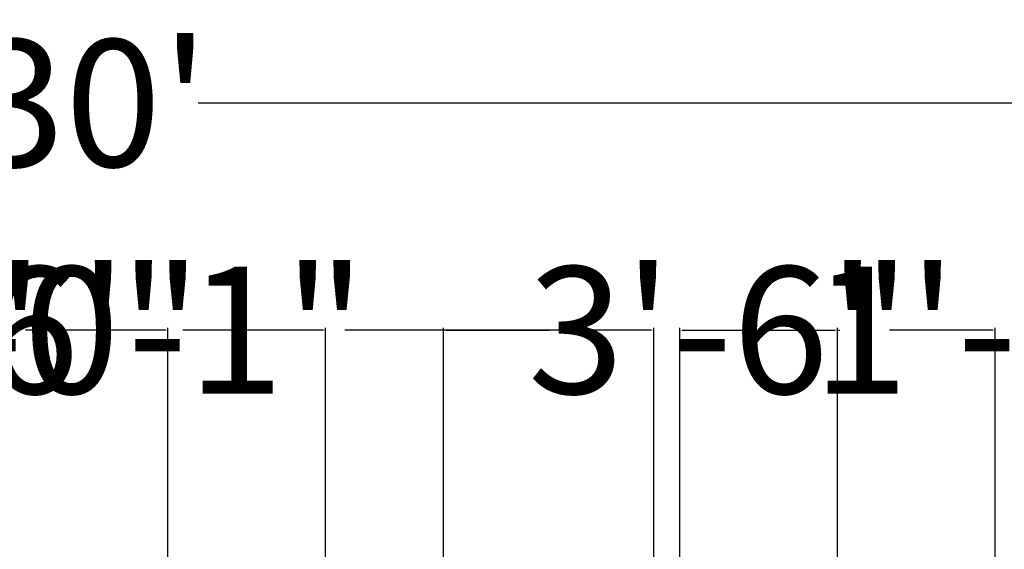
# Model space of a CAD drawing. Units: inches. Extents: x 2103 to 2702, y 2405 to 3142.
# Tile 5 of 7: x 2421 to 2496, y 3102 to 3142. Entities that reach past the tile are written whole.
import ezdxf

# ---------------------------------------------------------------- set-up
doc = ezdxf.new("R2010")
doc.units = ezdxf.units.IN
doc.layers.add('A-ANNO-DIMS', color=2, linetype='Continuous', lineweight=18)
doc.styles.get("Standard").update_dxf_attribs({"font": 'arial.ttf'})
doc.dimstyles.get("Standard").update_dxf_attribs({"dimtxt": 9.68, "dimasz": 0.18, "dimexe": 0.18, "dimexo": 0.0625, "dimgap": 0.09, "dimtad": 0, "dimtih": 1, "dimtoh": 1, "dimdec": 1, "dimzin": 0, "dimdsep": 46, "dimlunit": 3, "dimtxsty": 'Standard', "dimcen": 0.09, "dimadec": 0, "dimazin": 0, "dimtfac": 1, "dimtdec": 1, "dimtofl": 0, "dimtmove": 0, "dimatfit": 3, "dimfxl": 1, "dimtolj": 1, "dimtzin": 0, "dimarcsym": 0})

# ---------------------------------------------------------------- blocks, each defined once
blk = doc.blocks.new('*D15')
at = {"layer": 'A-ANNO-DIMS', "color": 0, "lineweight": -2, "transparency": 16777216}
for p, q in [((2246.430135310188, 3068.908174366427), (2246.430135310188, 3136.18297836625)), ((2606.430135310187, 3068.908174366427), (2606.430135310187, 3136.18297836625)), ((2246.610135310187, 3136.002978366251), (2418.129303113734, 3136.002978366251)), ((2606.250135310188, 3136.002978366251), (2434.730967506641, 3136.002978366251))]:
    blk.add_line(p, q, dxfattribs=at)
at = {"layer": 'A-ANNO-DIMS', "color": 0, "transparency": 16777216}
for points in [[(2246.610135310187, 3136.032978366251), (2246.610135310187, 3135.97297836625), (2246.430135310188, 3136.002978366251)], [(2606.250135310188, 3136.032978366251), (2606.250135310188, 3135.97297836625), (2606.430135310187, 3136.002978366251)]]:
    blk.add_solid(points, dxfattribs=at)
at = {"layer": 'Defpoints', "color": 0, "transparency": 16777216}
for p in [(2606.430135310187, 3136.002978366251), (2246.430135310188, 3068.845674366427), (2606.430135310187, 3068.845674366427)]:
    blk.add_point(p, dxfattribs=at)
at = {"layer": 'A-ANNO-DIMS', "color": 0, "transparency": 16777216, "insert": (2426.430135310188, 3136.002978366251), "char_height": 9.68, "attachment_point": 5}
blk.add_mtext("\\A1;30'", dxfattribs=at)
blk = doc.blocks.new('*D32')
at = {"layer": 'A-ANNO-DIMS', "color": 0, "lineweight": -2, "transparency": 16777216}
for p, q in [((2523.701954441973, 3069.816092044852), (2527.298623542507, 3072.777740503555)), ((2527.0452500719, 3072.802273835842), (2526.8652500719, 3072.802273835842)), ((2527.15967014106, 3072.663320434396), (2527.0452500719, 3072.802273835842)), ((2546.291633940058, 3049.429184449692), (2527.274090210219, 3072.524367032949)), ((2542.948338310131, 3046.443002658702), (2546.545007410664, 3049.404651117404))]:
    blk.add_line(p, q, dxfattribs=at)
at = {"layer": 'A-ANNO-DIMS', "color": 0, "transparency": 16777216}
for points in [[(2527.297249110461, 3072.543437044476), (2527.250931309978, 3072.505297021422), (2527.15967014106, 3072.663320434396)], [(2546.3147928403, 3049.448254461218), (2546.268475039817, 3049.410114438165), (2546.406054009218, 3049.290231048245)]]:
    blk.add_solid(points, dxfattribs=at)
at = {"layer": 'Defpoints', "color": 0, "transparency": 16777216}
for p in [(2527.15967014106, 3072.663320434396), (2523.653706733137, 3069.776362854172), (2542.900090601295, 3046.403273468022)]:
    blk.add_point(p, dxfattribs=at)
at = {"layer": 'A-ANNO-DIMS', "color": 0, "transparency": 16777216, "insert": (2430.028074082815, 3072.802273835842), "char_height": 9.68, "attachment_point": 5}
blk.add_mtext('\\A1;SINK ENVELOPE 2\'-6 1/2" TYP.', dxfattribs=at)
blk = doc.blocks.new('*D40')
at = {"layer": 'A-ANNO-DIMS', "color": 0, "lineweight": -2, "transparency": 16777216}
for p, q in [((2396.430135, 2906.908174), (2396.430135, 3118.895223)), ((2396.610135, 3118.715223000001), (2407.279400801501, 3118.715223000001)), ((2444.25014, 3118.715223000001), (2433.580874198499, 3118.715223000001)), ((2444.43014, 2842.908175), (2444.43014, 3118.895223))]:
    blk.add_line(p, q, dxfattribs=at)
at = {"layer": 'A-ANNO-DIMS', "color": 0, "transparency": 16777216}
for points in [[(2396.610135, 3118.745223000001), (2396.610135, 3118.685223), (2396.430135, 3118.715223000001)], [(2444.25014, 3118.745223000001), (2444.25014, 3118.685223), (2444.43014, 3118.715223000001)]]:
    blk.add_solid(points, dxfattribs=at)
at = {"layer": 'Defpoints', "color": 0, "transparency": 16777216}
for p in [(2444.43014, 3118.715223000001), (2396.430135, 2906.845674), (2444.43014, 2842.845675)]:
    blk.add_point(p, dxfattribs=at)
at = {"layer": 'A-ANNO-DIMS', "color": 0, "transparency": 16777216, "insert": (2420.4301375, 3118.715223000001), "char_height": 9.68, "attachment_point": 5}
blk.add_mtext('\\A1;4\'-0"', dxfattribs=at)
blk = doc.blocks.new('*D44')
at = {"layer": 'A-ANNO-DIMS', "color": 0, "lineweight": -2, "transparency": 16777216}
for p, q in [((2471.430135, 2560.908174), (2471.430135, 3118.895223)), ((2471.610135, 3118.715223000001), (2483.250135, 3118.715223000001)), ((2483.430135, 2560.908174), (2483.430135, 3118.895223)), ((2483.430135, 3118.715223000001), (2483.610135, 3118.715223000001))]:
    blk.add_line(p, q, dxfattribs=at)
at = {"layer": 'A-ANNO-DIMS', "color": 0, "transparency": 16777216}
for points in [[(2471.610135, 3118.745223000001), (2471.610135, 3118.685223), (2471.430135, 3118.715223000001)], [(2483.250135, 3118.745223000001), (2483.250135, 3118.685223), (2483.430135, 3118.715223000001)]]:
    blk.add_solid(points, dxfattribs=at)
at = {"layer": 'Defpoints', "color": 0, "transparency": 16777216}
for p in [(2483.430135, 3118.715223000001), (2471.430135, 2560.845674), (2483.430135, 2560.845674)]:
    blk.add_point(p, dxfattribs=at)
at = {"layer": 'A-ANNO-DIMS', "color": 0, "transparency": 16777216, "insert": (2496.11047606412, 3118.715223000001), "char_height": 9.68, "attachment_point": 5}
blk.add_mtext('\\A1;1\'-0"', dxfattribs=at)
blk = doc.blocks.new('*D50')
at = {"layer": 'A-ANNO-DIMS', "color": 0, "lineweight": -2, "transparency": 16777216}
for p, q in [((2453.430135, 2569.908174), (2453.430135, 3118.895223)), ((2453.610135, 3118.715223000001), (2461.477488342429, 3118.715223000001)), ((2495.250135, 3118.715223000001), (2487.382781657572, 3118.715223000001)), ((2495.430135, 2569.908174), (2495.430135, 3118.895223))]:
    blk.add_line(p, q, dxfattribs=at)
at = {"layer": 'A-ANNO-DIMS', "color": 0, "transparency": 16777216}
for points in [[(2453.610135, 3118.745223000001), (2453.610135, 3118.685223), (2453.430135, 3118.715223000001)], [(2495.250135, 3118.745223000001), (2495.250135, 3118.685223), (2495.430135, 3118.715223000001)]]:
    blk.add_solid(points, dxfattribs=at)
at = {"layer": 'Defpoints', "color": 0, "transparency": 16777216}
for p in [(2495.430135, 3118.715223000001), (2453.430135, 2569.845674), (2495.430135, 2569.845674)]:
    blk.add_point(p, dxfattribs=at)
at = {"layer": 'A-ANNO-DIMS', "color": 0, "transparency": 16777216, "insert": (2474.430135, 3118.715223000001), "char_height": 9.68, "attachment_point": 5}
blk.add_mtext('\\A1;3\'-6"', dxfattribs=at)
blk = doc.blocks.new('*D64')
at = {"layer": 'A-ANNO-DIMS', "color": 0, "lineweight": -2, "transparency": 16777216}
for p, q in [((2396.430135, 3059.908174), (2396.430135, 3118.895223)), ((2396.610135, 3118.715223000001), (2419.947774836289, 3118.715223000001)), ((2469.250135000001, 3118.715223000001), (2445.912495163711, 3118.715223000001)), ((2469.430135, 3059.908174), (2469.430135, 3118.895223))]:
    blk.add_line(p, q, dxfattribs=at)
at = {"layer": 'A-ANNO-DIMS', "color": 0, "transparency": 16777216}
for points in [[(2396.610135, 3118.745223000001), (2396.610135, 3118.685223), (2396.430135, 3118.715223000001)], [(2469.250135000001, 3118.745223000001), (2469.250135000001, 3118.685223), (2469.430135, 3118.715223000001)]]:
    blk.add_solid(points, dxfattribs=at)
at = {"layer": 'Defpoints', "color": 0, "transparency": 16777216}
for p in [(2469.430135, 3118.715223000001), (2396.430135, 3059.845674), (2469.430135, 3059.845674)]:
    blk.add_point(p, dxfattribs=at)
at = {"layer": 'A-ANNO-DIMS', "color": 0, "transparency": 16777216, "insert": (2432.930135, 3118.715223000001), "char_height": 9.68, "attachment_point": 5}
blk.add_mtext('\\A1;6\'-1"', dxfattribs=at)
blk = doc.blocks.new('*D66')
at = {"layer": 'A-ANNO-DIMS', "color": 0, "lineweight": -2, "transparency": 16777216}
for p, q in [((2384.430135, 2794.908174), (2384.430135, 3118.895223)), ((2384.610135, 3118.715223000001), (2395.279398301501, 3118.715223000001)), ((2432.250135, 3118.715223000001), (2421.5808716985, 3118.715223000001)), ((2432.430135000001, 2794.908174), (2432.430135000001, 3118.895223))]:
    blk.add_line(p, q, dxfattribs=at)
at = {"layer": 'A-ANNO-DIMS', "color": 0, "transparency": 16777216}
for points in [[(2384.610135, 3118.745223000001), (2384.610135, 3118.685223), (2384.430135, 3118.715223000001)], [(2432.250135, 3118.745223000001), (2432.250135, 3118.685223), (2432.430135000001, 3118.715223000001)]]:
    blk.add_solid(points, dxfattribs=at)
at = {"layer": 'Defpoints', "color": 0, "transparency": 16777216}
for p in [(2384.430135, 3118.715223000001), (2384.430135, 2794.845674), (2432.430135000001, 2794.845674)]:
    blk.add_point(p, dxfattribs=at)
at = {"layer": 'A-ANNO-DIMS', "color": 0, "transparency": 16777216, "insert": (2408.430135, 3118.715223000001), "char_height": 9.68, "attachment_point": 5}
blk.add_mtext('\\A1;4\'-0"', dxfattribs=at)

msp = doc.modelspace()

# ---------------------------------------------------------------- dimensions: what is measured, and where the dimension line sits
at = {"layer": 'A-ANNO-DIMS'}
for base, p1, p2, override, picture, middle in [((2606.430135310187, 3136.002978366251), (2246.430135310188, 3068.845674366427), (2606.430135310187, 3068.845674366427), {"dimclrd": 0, "dimclre": 0, "dimclrt": 0}, '*D15', (2426.430135310188, 3136.002978366251)), ((2384.430135, 3118.715223000001), (2432.430135000001, 2794.845674), (2384.430135, 2794.845674), {"dimdec": 1, "dimlfac": 1, "dimrnd": 0, "dimzin": 1, "dimdsep": 46, "dimlunit": 4, "dimfrac": 2}, '*D66', (2408.430135, 3118.715223000001)), ((2444.43014, 3118.715223000001), (2396.430135, 2906.845674), (2444.43014, 2842.845675), {"dimdec": 1, "dimlfac": 1, "dimrnd": 0, "dimzin": 1, "dimdsep": 46, "dimlunit": 4, "dimfrac": 2}, '*D40', (2420.4301375, 3118.715223000001)), ((2469.430135, 3118.715223000001), (2396.430135, 3059.845674), (2469.430135, 3059.845674), {"dimdec": 1, "dimlfac": 1, "dimrnd": 0, "dimzin": 1, "dimdsep": 46, "dimlunit": 4, "dimfrac": 2}, '*D64', (2432.930135, 3118.715223000001)), ((2495.430135, 3118.715223000001), (2453.430135, 2569.845674), (2495.430135, 2569.845674), {"dimdec": 1, "dimlfac": 1, "dimrnd": 0, "dimzin": 1, "dimdsep": 46, "dimlunit": 4, "dimfrac": 2}, '*D50', (2474.430135, 3118.715223000001)), ((2483.430135, 3118.715223000001), (2471.430135, 2560.845674), (2483.430135, 2560.845674), {"dimdec": 1, "dimlfac": 1, "dimrnd": 0, "dimzin": 1, "dimdsep": 46, "dimlunit": 4, "dimfrac": 2}, '*D44', (2496.11047606412, 3118.715223000001))]:
    dim = msp.add_linear_dim(base=base, p1=p1, p2=p2, dimstyle='Standard', override=override, dxfattribs=at)
    dim.commit()
    dim.dimension.update_dxf_attribs({"geometry": picture, "text_midpoint": middle})
dim = msp.add_linear_dim(base=(2527.15967014106, 3072.663320434396), p1=(2542.900090601295, 3046.403273468023), p2=(2523.653706733138, 3069.776362854172), angle=129.4694759592849, text='SINK ENVELOPE <> TYP.', dimstyle='Standard', override={"dimdec": 1, "dimlfac": 1, "dimrnd": 0, "dimzin": 1, "dimdsep": 46, "dimlunit": 4, "dimfrac": 2}, dxfattribs=at)
dim.commit()
dim.dimension.update_dxf_attribs({"geometry": '*D32', "text_midpoint": (2430.028074082815, 3072.802273835842)})

doc.saveas('drawing.dxf')
